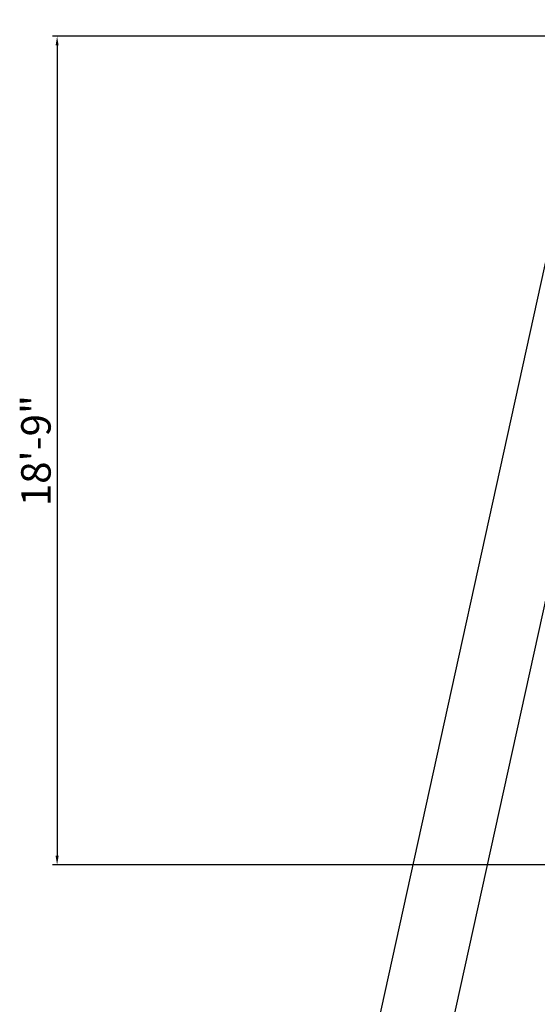
# Model space of a CAD drawing. Units: inches. Extents: x 2642 to 4124, y 1227 to 1973.
# Tile 4 of 7: x 3343 to 3483, y 1645 to 1912. Entities that reach past the tile are written whole.
import ezdxf

# ---------------------------------------------------------------- set-up
doc = ezdxf.new("R2010")
doc.units = ezdxf.units.IN
doc.layers.add('A-ANNO-DIMS', color=2, linetype='Continuous', lineweight=18)
doc.layers.add('C-PROP', color=7, linetype='Continuous', lineweight=25)
doc.styles.get("Standard").update_dxf_attribs({"font": 'arial.ttf'})
doc.dimstyles.new('ISO-25', dxfattribs={"dimtxt": 8, "dimasz": 2.5, "dimexe": 1.25, "dimexo": 0.625, "dimtad": 1, "dimdec": 0, "dimlunit": 3, "dimtxsty": 'Standard', "dimcen": 2.5, "dimadec": 0, "dimazin": 0, "dimtfac": 1, "dimtdec": 0, "dimtmove": 0, "dimatfit": 3, "dimfxl": 1, "dimarcsym": 0})

# ---------------------------------------------------------------- blocks, each defined once
blk = doc.blocks.new('*D4')
at = {"layer": 'A-ANNO-DIMS', "color": 0, "lineweight": -2, "transparency": 16777216}
for p, q in [((3518.61, 1907.92), (3498.8, 1912.28)), ((3368.56, 1314.45), (3499.49, 1909.57)), ((3386.61, 1307.92), (3366.8, 1312.28))]:
    blk.add_line(p, q, dxfattribs=at)
at = {"layer": 'A-ANNO-DIMS', "color": 0, "transparency": 16777216}
for points in [[(3499.08, 1909.65), (3499.89, 1909.48), (3500.02, 1912.01)], [(3368.15, 1314.54), (3368.97, 1314.36), (3368.02, 1312.01)]]:
    blk.add_solid(points, dxfattribs=at)
at = {"layer": 'Defpoints', "color": 0, "transparency": 16777216}
for p in [(3500.02, 1912.01), (3519.22, 1907.78), (3387.22, 1307.78)]:
    blk.add_point(p, dxfattribs=at)
at = {"layer": 'A-ANNO-DIMS', "color": 0, "transparency": 16777216, "insert": (3429.42, 1613.02), "char_height": 8, "attachment_point": 5, "rotation": 77.5926}
blk.add_mtext('51\'-2"', dxfattribs=at)
blk = doc.blocks.new('*D70')
at = {"layer": 'A-ANNO-DIMS', "color": 0, "lineweight": -2, "transparency": 16777216}
for p, q in [((3518.6, 1907.78), (3351.67, 1907.78)), ((3352.92, 1905.28), (3352.92, 1685.28)), ((3485.6, 1682.78), (3351.67, 1682.78))]:
    blk.add_line(p, q, dxfattribs=at)
at = {"layer": 'A-ANNO-DIMS', "color": 0, "transparency": 16777216}
for points in [[(3352.51, 1905.28), (3353.34, 1905.28), (3352.92, 1907.78)], [(3352.51, 1685.28), (3353.34, 1685.28), (3352.92, 1682.78)]]:
    blk.add_solid(points, dxfattribs=at)
at = {"layer": 'Defpoints', "color": 0, "transparency": 16777216}
for p in [(3519.22, 1907.78), (3352.92, 1682.78), (3486.22, 1682.78)]:
    blk.add_point(p, dxfattribs=at)
at = {"layer": 'A-ANNO-DIMS', "color": 0, "transparency": 16777216, "insert": (3348.21, 1795.28), "char_height": 8, "attachment_point": 5, "rotation": 90}
blk.add_mtext('18\'-9"', dxfattribs=at)

msp = doc.modelspace()

# ---------------------------------------------------------------- linework, layer by layer
at = {"layer": 'C-PROP'}
msp.add_line((3519.22, 1907.78), (3387.22, 1307.78), dxfattribs=at)

# ---------------------------------------------------------------- dimensions: what is measured, and where the dimension line sits
at = {"layer": 'A-ANNO-DIMS'}
dim = msp.add_aligned_dim(p1=(3387.22, 1307.78), p2=(3519.22, 1907.78), distance=19.66, dimstyle='ISO-25', override={"dimclrd": 0, "dimclre": 0, "dimclrt": 0}, dxfattribs=at)
dim.commit()
dim.dimension.update_dxf_attribs({"geometry": '*D4', "text_midpoint": (3429.42, 1613.02)})
dim = msp.add_linear_dim(base=(3352.92, 1682.78), p1=(3519.22, 1907.78), p2=(3486.22, 1682.78), angle=90, dimstyle='ISO-25', override={"dimdec": 1, "dimlfac": 1, "dimrnd": 0, "dimzin": 1, "dimdsep": 46, "dimlunit": 4, "dimfrac": 2}, dxfattribs=at)
dim.commit()
dim.dimension.update_dxf_attribs({"geometry": '*D70', "text_midpoint": (3348.21, 1795.28)})

doc.saveas('drawing.dxf')
